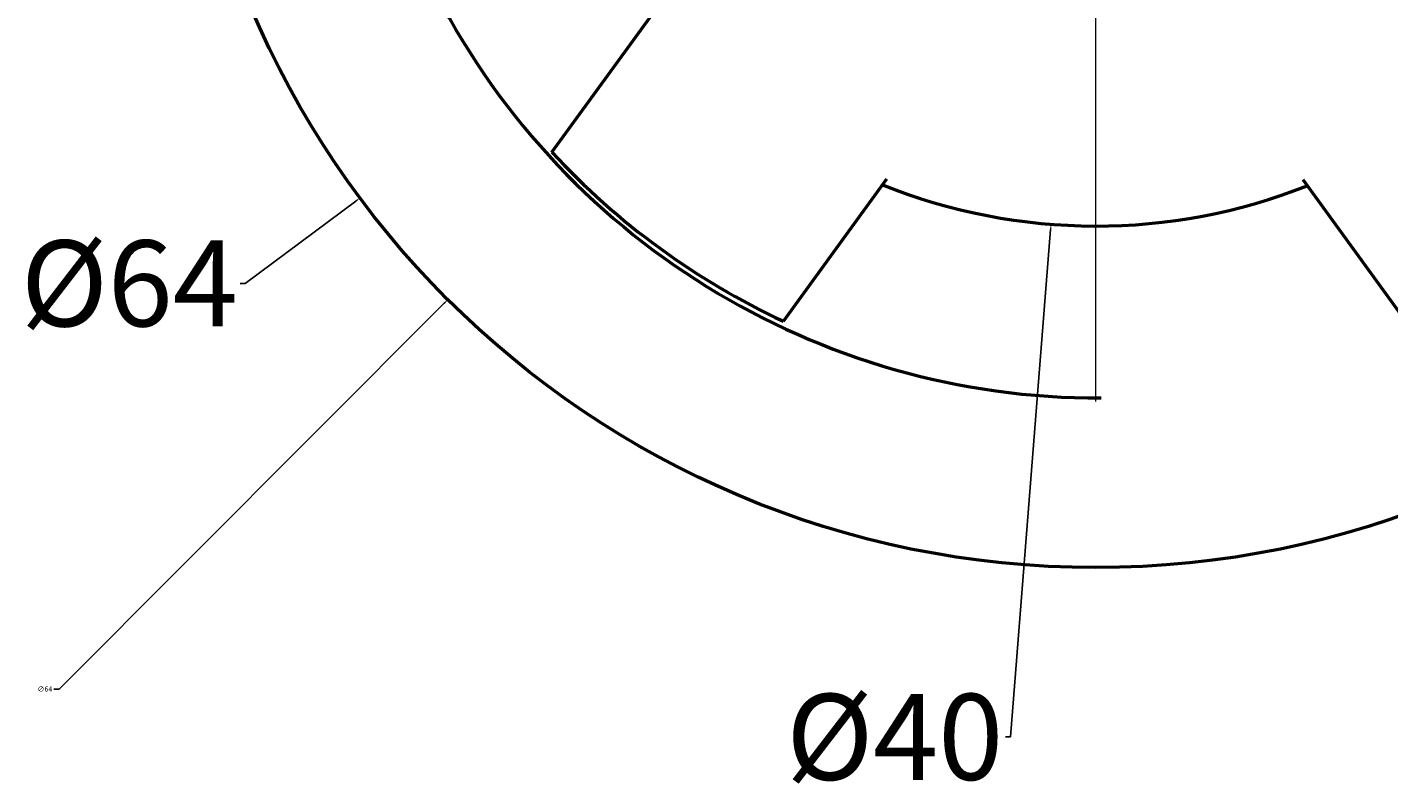
# Model space of a CAD drawing. Units: millimetres. Extents: x -50 to 109, y -46 to 152.
# Tile 1 of 18: x -38 to 9, y -46 to -20. Entities that reach past the tile are written whole.
import ezdxf

# ---------------------------------------------------------------- set-up
doc = ezdxf.new("R2010")
doc.units = ezdxf.units.MM
doc.header["$MEASUREMENT"] = 0
doc.linetypes.add('CENTER', pattern=[50.8, 31.75, -6.35, 6.35, -6.35])
for name, color, linetype, lineweight in [('M-CNTR', 1, 'CENTER', 18), ('M-DIMS', 2, 'Continuous', 25), ('M-OUTL', 7, 'Continuous', 50)]:
    doc.layers.add(name, color=color, linetype=linetype, lineweight=lineweight)
doc.styles.get("Standard").update_dxf_attribs({"font": 'arial.ttf'})
doc.dimstyles.get("Standard").update_dxf_attribs({"dimtxt": 0.18, "dimasz": 0.18, "dimexe": 0.18, "dimexo": 0.0625, "dimgap": 0.09, "dimtad": 0, "dimtih": 1, "dimtoh": 1, "dimdec": 4, "dimzin": 0, "dimdsep": 46, "dimtxsty": 'Standard', "dimcen": 0.09, "dimadec": 0, "dimazin": 0, "dimtfac": 1, "dimtdec": 4, "dimtofl": 0, "dimtmove": 0, "dimatfit": 3, "dimfxl": 1, "dimtolj": 1, "dimtzin": 0, "dimarcsym": 0})

# ---------------------------------------------------------------- blocks, each defined once
blk = doc.blocks.new('*U1')
for p, q in [((-5, 2.851), (-5, -3.294)), ((5, 2.824), (5, -3.323))]:
    blk.add_line(p, q)
blk.add_arc((-0.069, -22.677), 26, 78.7582, 100.9333)
blk = doc.blocks.new('*U2')
at = {"layer": 'M-OUTL', "color": 0, "linetype": 'ByBlock', "lineweight": -2, "transparency": 16777216}
blk.add_blockref('*U1', (-0.855, 15.809), dxfattribs=at)
for p, rotation in [((-22.328, 0.278), 72), ((20.551, 0.185), 288), ((-14.194, -24.943), 144), ((12.307, -25), 216)]:
    blk.add_blockref('*U1', p, dxfattribs=dict(at, rotation=rotation))
blk = doc.blocks.new('*U6')
at = {"layer": 'M-CNTR', "color": 0, "transparency": 16777216}
for p, q in [((0, 5.2), (0, 36)), ((-26.12, 0), (-5.2, 0)), ((5.2, 0), (26.12, 0)), ((0, -26.12), (0, -5.2))]:
    blk.add_line(p, q, dxfattribs=at)
at = {"layer": 'M-CNTR', "color": 0, "linetype": 'Continuous', "transparency": 16777216}
for p, q in [((0, -2.6), (0, 2.6)), ((-2.6, 0), (2.6, 0))]:
    blk.add_line(p, q, dxfattribs=at)
blk = doc.blocks.new('*D22')
at = {"layer": 'Defpoints', "color": 0, "transparency": 16777216}
for p in [(0.661, 13.074), (-2.483, -26.803)]:
    blk.add_point(p, dxfattribs=at)
at = {"layer": 'M-DIMS', "color": 0, "lineweight": -2, "transparency": 16777216}
for p, q in [((-1.001, -6.864), (-0.821, -6.864)), ((-0.911, -6.954), (-0.911, -6.774)), ((-3.894, -44.69), (-2.498, -26.982)), ((-4.074, -44.69), (-3.894, -44.69))]:
    blk.add_line(p, q, dxfattribs=at)
at = {"layer": 'M-DIMS', "color": 0, "transparency": 16777216}
blk.add_solid([(-2.527, -26.98), (-2.468, -26.984), (-2.483, -26.803)], dxfattribs=at)
at = {"layer": 'M-DIMS', "color": 0, "transparency": 16777216, "insert": (-7.94, -44.69), "char_height": 0.18, "attachment_point": 5}
blk.add_mtext('\\A1;{\\H16.66667x;%%C40}', dxfattribs=at)
blk = doc.blocks.new('*D23')
at = {"layer": 'Defpoints', "color": 0, "transparency": 16777216}
for p in [(24.75, 12.317), (-26.598, -25.885)]:
    blk.add_point(p, dxfattribs=at)
at = {"layer": 'M-DIMS', "color": 0, "lineweight": -2, "transparency": 16777216}
for p, q in [((-1.014, -6.784), (-0.834, -6.784)), ((-0.924, -6.874), (-0.924, -6.694)), ((-30.604, -28.865), (-26.742, -25.992)), ((-30.784, -28.865), (-30.604, -28.865))]:
    blk.add_line(p, q, dxfattribs=at)
at = {"layer": 'M-DIMS', "color": 0, "transparency": 16777216}
blk.add_solid([(-26.76, -25.968), (-26.724, -26.016), (-26.598, -25.885)], dxfattribs=at)
at = {"layer": 'M-DIMS', "color": 0, "transparency": 16777216, "insert": (-34.648, -28.865), "char_height": 0.18, "attachment_point": 5}
blk.add_mtext('\\A1;{\\H16.66667x;%%C64}', dxfattribs=at)
blk = doc.blocks.new('*D24')
at = {"layer": 'Defpoints', "color": 0, "transparency": 16777216}
for p in [(-9.958, 17.477), (8.318, -31.205)]:
    blk.add_point(p, dxfattribs=at)
at = {"layer": 'M-DIMS', "color": 0, "lineweight": -2, "transparency": 16777216}
for p, q in [((-13.793, 27.212), (-13.613, 27.212)), ((-13.613, 27.212), (-10.022, 17.646)), ((-0.91, -6.864), (-0.73, -6.864)), ((-0.82, -6.954), (-0.82, -6.774))]:
    blk.add_line(p, q, dxfattribs=at)
at = {"layer": 'M-DIMS', "color": 0, "transparency": 16777216}
blk.add_solid([(-9.994, 17.656), (-10.05, 17.635), (-9.958, 17.477)], dxfattribs=at)
at = {"layer": 'M-DIMS', "color": 0, "transparency": 16777216, "insert": (-17.649, 27.212), "char_height": 0.18, "attachment_point": 5}
blk.add_mtext('\\A1;{\\H16.66667x;%%C52}', dxfattribs=at)
blk = doc.blocks.new('*D29')
at = {"layer": 'Defpoints', "color": 0, "transparency": 16777216}
for p in [(21.684, 15.863), (-23.531, -29.431)]:
    blk.add_point(p, dxfattribs=at)
at = {"layer": 'M-DIMS', "color": 0, "lineweight": -2, "transparency": 16777216}
for p, q in [((-1.014, -6.784), (-0.834, -6.784)), ((-0.924, -6.874), (-0.924, -6.694)), ((-37.096, -43.02), (-23.658, -29.559)), ((-37.276, -43.02), (-37.096, -43.02))]:
    blk.add_line(p, q, dxfattribs=at)
at = {"layer": 'M-DIMS', "color": 0, "transparency": 16777216}
blk.add_solid([(-23.68, -29.537), (-23.637, -29.58), (-23.531, -29.431)], dxfattribs=at)
at = {"layer": 'M-DIMS', "color": 0, "transparency": 16777216, "insert": (-37.592, -43.02), "char_height": 0.18, "attachment_point": 5}
blk.add_mtext('\\A1;∅64', dxfattribs=at)

msp = doc.modelspace()

# ---------------------------------------------------------------- linework, layer by layer
at = {"layer": 'M-OUTL'}
msp.add_circle((-0.92366, -6.78396), 32, dxfattribs=at)
for centre, radius, start, end in [((-0.82008, -6.86387), 26, 78.565718, 270.188748), ((-0.91099, -6.86447), 20, 248.123165, 291.621046)]:
    msp.add_arc(centre, radius, start, end, dxfattribs=at)

# ---------------------------------------------------------------- block references
at = {"layer": 'M-CNTR'}
msp.add_blockref('*U6', (-0.92366, -6.86889), dxfattribs=at)
at = {"layer": 'M-OUTL'}
msp.add_blockref('*U2', (0, 0), dxfattribs=at)

# ---------------------------------------------------------------- dimensions: what is measured, and where the dimension line sits
at = {"layer": 'M-DIMS'}
for p1, p2, text, picture, middle in [((8.31828, -31.20499), (-9.95844, 17.47726), '{\\H16.66667x;%%C52}', '*D24', (-17.64865, 27.21244)), ((0.6614, 13.07362), (-2.48337, -26.80257), '{\\H16.66667x;%%C40}', '*D22', (-7.93965, -44.69043)), ((24.75033, 12.31698), (-26.59765, -25.88491), '{\\H16.66667x;%%C64}', '*D23', (-34.64806, -28.86518))]:
    dim = msp.add_diameter_dim_2p(p1=p1, p2=p2, text=text, dimstyle='Standard', override={"dimclrd": 0, "dimclre": 0, "dimclrt": 0}, dxfattribs=at)
    dim.commit()
    dim.dimension.update_dxf_attribs({"geometry": picture, "text_midpoint": middle, "dimtype": 163})
dim = msp.add_diameter_dim_2p(p1=(21.68387, 15.86332), p2=(-23.53119, -29.43125), dimstyle='Standard', override={"dimdec": 0, "dimlfac": 1, "dimrnd": 0, "dimzin": 0, "dimdsep": 46, "dimlunit": 2}, dxfattribs=at)
dim.commit()
dim.dimension.update_dxf_attribs({"geometry": '*D29', "text_midpoint": (-37.59218, -43.01962), "dimtype": 163})

doc.saveas('drawing.dxf')
